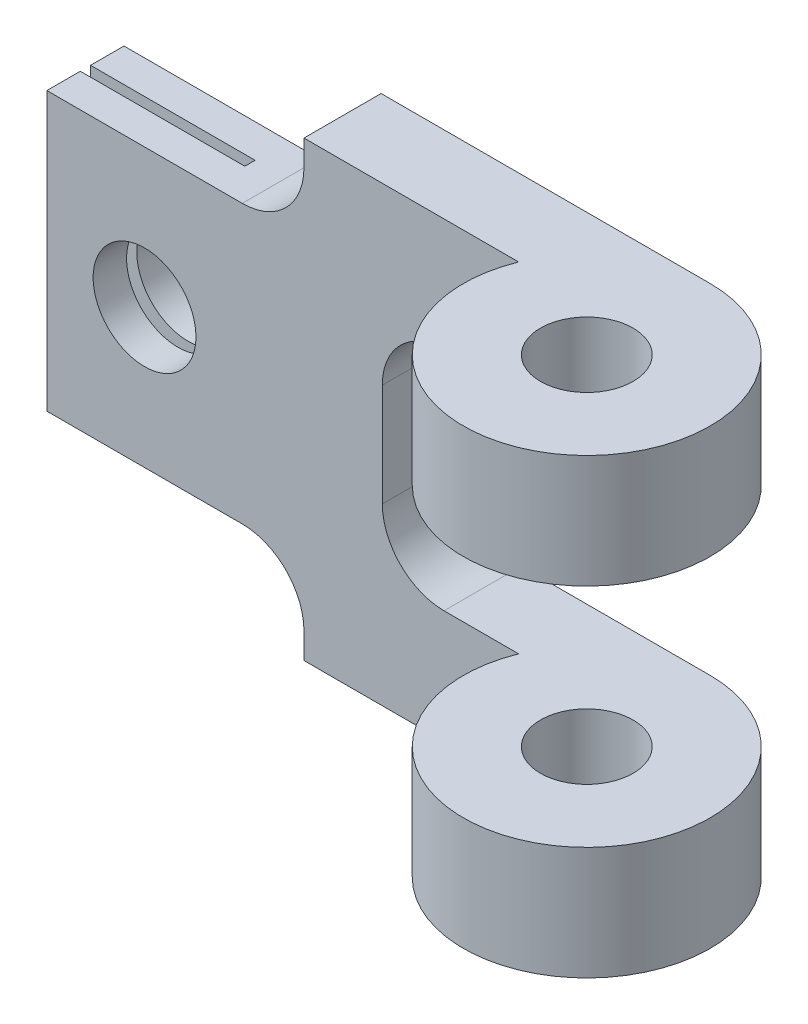
ISO-10303-21;
HEADER;
FILE_DESCRIPTION(('STEP AP214'),'2;1');
FILE_NAME('part.step','',(''),(''),'','','');
FILE_SCHEMA(('AUTOMOTIVE_DESIGN { 1 0 10303 214 1 1 1 1 }'));
ENDSEC;
DATA;
#1=APPLICATION_CONTEXT('core data for automotive mechanical design processes');
#2=APPLICATION_PROTOCOL_DEFINITION('international standard','automotive_design',2000,#1);
#3=PRODUCT_CONTEXT('',#1,'mechanical');
#4=PRODUCT('Part','Part','',(#3));
#5=PRODUCT_RELATED_PRODUCT_CATEGORY('part','',(#4));
#6=PRODUCT_DEFINITION_FORMATION('','',#4);
#7=PRODUCT_DEFINITION_CONTEXT('part definition',#1,'design');
#8=PRODUCT_DEFINITION('design','',#6,#7);
#9=PRODUCT_DEFINITION_SHAPE('','',#8);
#10=(LENGTH_UNIT() NAMED_UNIT(*) SI_UNIT(.MILLI.,.METRE.));
#11=(NAMED_UNIT(*) PLANE_ANGLE_UNIT() SI_UNIT($,.RADIAN.));
#12=(NAMED_UNIT(*) SI_UNIT($,.STERADIAN.) SOLID_ANGLE_UNIT());
#13=UNCERTAINTY_MEASURE_WITH_UNIT(LENGTH_MEASURE(1.E-05),#10,'distance_accuracy_value','');
#14=(GEOMETRIC_REPRESENTATION_CONTEXT(3) GLOBAL_UNCERTAINTY_ASSIGNED_CONTEXT((#13)) GLOBAL_UNIT_ASSIGNED_CONTEXT((#10,
#11,#12)) REPRESENTATION_CONTEXT('',''));
#15=CARTESIAN_POINT('',(0.,0.,0.));
#16=DIRECTION('',(0.,0.,1.));
#17=DIRECTION('',(1.,0.,0.));
#18=AXIS2_PLACEMENT_3D('',#15,#16,#17);
#19=CARTESIAN_POINT('',(-50.,-71.,15.));
#20=DIRECTION('',(-1.,0.,0.));
#21=DIRECTION('',(0.,0.,1.));
#22=AXIS2_PLACEMENT_3D('',#19,#20,#21);
#23=PLANE('',#22);
#24=DIRECTION('',(0.,1.,0.));
#25=VECTOR('',#24,1.);
#26=CARTESIAN_POINT('',(-50.,-72.,6.5));
#27=LINE('',#26,#25);
#28=CARTESIAN_POINT('',(-50.,-71.,6.5));
#29=VERTEX_POINT('',#28);
#30=CARTESIAN_POINT('',(-50.,-17.,6.5));
#31=VERTEX_POINT('',#30);
#32=EDGE_CURVE('E330',#29,#31,#27,.T.);
#33=ORIENTED_EDGE('',*,*,#32,.T.);
#34=DIRECTION('',(0.,0.,-1.));
#35=VECTOR('',#34,1.);
#36=CARTESIAN_POINT('',(-50.,-17.,15.));
#37=LINE('',#36,#35);
#38=CARTESIAN_POINT('',(-50.,-17.,0.));
#39=VERTEX_POINT('',#38);
#40=EDGE_CURVE('E206',#31,#39,#37,.T.);
#41=ORIENTED_EDGE('',*,*,#40,.T.);
#42=DIRECTION('',(0.,1.,0.));
#43=VECTOR('',#42,1.);
#44=CARTESIAN_POINT('',(-50.,-71.,0.));
#45=LINE('',#44,#43);
#46=CARTESIAN_POINT('',(-50.,-71.,0.));
#47=VERTEX_POINT('',#46);
#48=EDGE_CURVE('E332',#47,#39,#45,.T.);
#49=ORIENTED_EDGE('',*,*,#48,.F.);
#50=DIRECTION('',(0.,0.,-1.));
#51=VECTOR('',#50,1.);
#52=CARTESIAN_POINT('',(-50.,-71.,15.));
#53=LINE('',#52,#51);
#54=EDGE_CURVE('E219',#29,#47,#53,.T.);
#55=ORIENTED_EDGE('',*,*,#54,.F.);
#56=EDGE_LOOP('',(#33,#41,#49,#55));
#57=FACE_BOUND('',#56,.T.);
#58=ADVANCED_FACE('F44',(#57),#23,.T.);
#59=CARTESIAN_POINT('',(0.,0.,15.));
#60=DIRECTION('',(1.,0.,0.));
#61=DIRECTION('',(0.,0.,-1.));
#62=AXIS2_PLACEMENT_3D('',#59,#60,#61);
#63=PLANE('',#62);
#64=DIRECTION('',(0.,0.,-1.));
#65=VECTOR('',#64,1.);
#66=CARTESIAN_POINT('',(0.,-83.0000000000001,15.));
#67=LINE('',#66,#65);
#68=CARTESIAN_POINT('',(0.,-83.,15.));
#69=VERTEX_POINT('',#68);
#70=CARTESIAN_POINT('',(0.,-83.0000000000001,0.));
#71=VERTEX_POINT('',#70);
#72=EDGE_CURVE('E218',#69,#71,#67,.T.);
#73=ORIENTED_EDGE('',*,*,#72,.T.);
#74=DIRECTION('',(0.,-1.,0.));
#75=VECTOR('',#74,1.);
#76=CARTESIAN_POINT('',(0.,0.,0.));
#77=LINE('',#76,#75);
#78=CARTESIAN_POINT('',(0.,-88.,0.));
#79=VERTEX_POINT('',#78);
#80=EDGE_CURVE('E239',#71,#79,#77,.T.);
#81=ORIENTED_EDGE('',*,*,#80,.T.);
#82=DIRECTION('',(0.,0.,-1.));
#83=VECTOR('',#82,1.);
#84=CARTESIAN_POINT('',(0.,-88.,15.));
#85=LINE('',#84,#83);
#86=CARTESIAN_POINT('',(0.,-88.,15.));
#87=VERTEX_POINT('',#86);
#88=EDGE_CURVE('E294',#87,#79,#85,.T.);
#89=ORIENTED_EDGE('',*,*,#88,.F.);
#90=DIRECTION('',(0.,-1.,0.));
#91=VECTOR('',#90,1.);
#92=CARTESIAN_POINT('',(0.,0.,15.));
#93=LINE('',#92,#91);
#94=EDGE_CURVE('E68',#69,#87,#93,.T.);
#95=ORIENTED_EDGE('',*,*,#94,.F.);
#96=EDGE_LOOP('',(#73,#81,#89,#95));
#97=FACE_BOUND('',#96,.T.);
#98=ADVANCED_FACE('F395',(#97),#63,.F.);
#99=CARTESIAN_POINT('',(0.,0.,0.));
#100=VERTEX_POINT('',#99);
#101=CARTESIAN_POINT('',(0.,-5.,0.));
#102=VERTEX_POINT('',#101);
#103=EDGE_CURVE('E256',#100,#102,#77,.T.);
#104=ORIENTED_EDGE('',*,*,#103,.T.);
#105=DIRECTION('',(0.,0.,-1.));
#106=VECTOR('',#105,1.);
#107=CARTESIAN_POINT('',(0.,-4.99999999999992,15.));
#108=LINE('',#107,#106);
#109=CARTESIAN_POINT('',(0.,-5.,15.));
#110=VERTEX_POINT('',#109);
#111=EDGE_CURVE('E208',#110,#102,#108,.T.);
#112=ORIENTED_EDGE('',*,*,#111,.F.);
#113=CARTESIAN_POINT('',(0.,0.,15.));
#114=VERTEX_POINT('',#113);
#115=EDGE_CURVE('E241',#114,#110,#93,.T.);
#116=ORIENTED_EDGE('',*,*,#115,.F.);
#117=DIRECTION('',(0.,0.,-1.));
#118=VECTOR('',#117,1.);
#119=CARTESIAN_POINT('',(0.,0.,15.));
#120=LINE('',#119,#118);
#121=EDGE_CURVE('E259',#114,#100,#120,.T.);
#122=ORIENTED_EDGE('',*,*,#121,.T.);
#123=EDGE_LOOP('',(#104,#112,#116,#122));
#124=FACE_BOUND('',#123,.T.);
#125=ADVANCED_FACE('F50',(#124),#63,.F.);
#126=CARTESIAN_POINT('',(0.,-88.,15.));
#127=DIRECTION('',(0.,1.,0.));
#128=DIRECTION('',(0.,0.,1.));
#129=AXIS2_PLACEMENT_3D('',#126,#127,#128);
#130=PLANE('',#129);
#131=CARTESIAN_POINT('',(64.,-88.,24.));
#132=DIRECTION('',(0.,1.,0.));
#133=DIRECTION('',(0.,0.,1.));
#134=AXIS2_PLACEMENT_3D('',#131,#132,#133);
#135=CIRCLE('',#134,9.);
#136=CARTESIAN_POINT('',(64.,-88.,33.));
#137=VERTEX_POINT('',#136);
#138=EDGE_CURVE('E412',#137,#137,#135,.T.);
#139=ORIENTED_EDGE('',*,*,#138,.T.);
#140=EDGE_LOOP('',(#139));
#141=FACE_BOUND('',#140,.T.);
#142=DIRECTION('',(1.,0.,0.));
#143=VECTOR('',#142,1.);
#144=CARTESIAN_POINT('',(0.,-88.,0.));
#145=LINE('',#144,#143);
#146=CARTESIAN_POINT('',(64.,-88.,0.));
#147=VERTEX_POINT('',#146);
#148=EDGE_CURVE('E264',#79,#147,#145,.T.);
#149=ORIENTED_EDGE('',*,*,#148,.T.);
#150=CARTESIAN_POINT('',(64.,-88.,24.));
#151=DIRECTION('',(0.,-1.,0.));
#152=DIRECTION('',(0.,0.,-1.));
#153=AXIS2_PLACEMENT_3D('',#150,#151,#152);
#154=CIRCLE('',#153,24.);
#155=CARTESIAN_POINT('',(41.751404538713,-88.,15.));
#156=VERTEX_POINT('',#155);
#157=EDGE_CURVE('E228',#147,#156,#154,.T.);
#158=ORIENTED_EDGE('',*,*,#157,.T.);
#159=DIRECTION('',(1.,0.,0.));
#160=VECTOR('',#159,1.);
#161=CARTESIAN_POINT('',(0.,-88.,15.));
#162=LINE('',#161,#160);
#163=EDGE_CURVE('E242',#87,#156,#162,.T.);
#164=ORIENTED_EDGE('',*,*,#163,.F.);
#165=ORIENTED_EDGE('',*,*,#88,.T.);
#166=EDGE_LOOP('',(#149,#158,#164,#165));
#167=FACE_BOUND('',#166,.T.);
#168=ADVANCED_FACE('F394',(#141,#167),#130,.F.);
#169=CARTESIAN_POINT('',(64.,-66.,15.));
#170=DIRECTION('',(0.,-1.,0.));
#171=DIRECTION('',(0.,0.,-1.));
#172=AXIS2_PLACEMENT_3D('',#169,#170,#171);
#173=PLANE('',#172);
#174=CARTESIAN_POINT('',(64.,-66.,24.));
#175=DIRECTION('',(0.,-1.,0.));
#176=DIRECTION('',(0.,0.,-1.));
#177=AXIS2_PLACEMENT_3D('',#174,#175,#176);
#178=CIRCLE('',#177,9.);
#179=CARTESIAN_POINT('',(64.,-66.,33.));
#180=VERTEX_POINT('',#179);
#181=EDGE_CURVE('E420',#180,#180,#178,.T.);
#182=ORIENTED_EDGE('',*,*,#181,.T.);
#183=EDGE_LOOP('',(#182));
#184=FACE_BOUND('',#183,.T.);
#185=CARTESIAN_POINT('',(64.,-66.,24.));
#186=DIRECTION('',(0.,-1.,0.));
#187=DIRECTION('',(0.,0.,-1.));
#188=AXIS2_PLACEMENT_3D('',#185,#186,#187);
#189=CIRCLE('',#188,24.);
#190=CARTESIAN_POINT('',(64.,-66.,0.));
#191=VERTEX_POINT('',#190);
#192=CARTESIAN_POINT('',(41.751404538713,-66.,15.));
#193=VERTEX_POINT('',#192);
#194=EDGE_CURVE('E224',#191,#193,#189,.T.);
#195=ORIENTED_EDGE('',*,*,#194,.F.);
#196=DIRECTION('',(-1.,0.,0.));
#197=VECTOR('',#196,1.);
#198=CARTESIAN_POINT('',(64.,-66.,0.));
#199=LINE('',#198,#197);
#200=CARTESIAN_POINT('',(27.2400000000001,-66.,0.));
#201=VERTEX_POINT('',#200);
#202=EDGE_CURVE('E267',#191,#201,#199,.T.);
#203=ORIENTED_EDGE('',*,*,#202,.T.);
#204=DIRECTION('',(0.,0.,-1.));
#205=VECTOR('',#204,1.);
#206=CARTESIAN_POINT('',(27.2400000000001,-66.,15.));
#207=LINE('',#206,#205);
#208=CARTESIAN_POINT('',(27.2400000000001,-66.,15.));
#209=VERTEX_POINT('',#208);
#210=EDGE_CURVE('E292',#209,#201,#207,.T.);
#211=ORIENTED_EDGE('',*,*,#210,.F.);
#212=DIRECTION('',(-1.,0.,0.));
#213=VECTOR('',#212,1.);
#214=CARTESIAN_POINT('',(64.,-66.,15.));
#215=LINE('',#214,#213);
#216=EDGE_CURVE('E246',#193,#209,#215,.T.);
#217=ORIENTED_EDGE('',*,*,#216,.F.);
#218=EDGE_LOOP('',(#195,#203,#211,#217));
#219=FACE_BOUND('',#218,.T.);
#220=ADVANCED_FACE('F389',(#184,#219),#173,.F.);
#221=CARTESIAN_POINT('',(27.24,-54.,15.));
#222=DIRECTION('',(0.,0.,-1.));
#223=DIRECTION('',(-1.,0.,0.));
#224=AXIS2_PLACEMENT_3D('',#221,#222,#223);
#225=CYLINDRICAL_SURFACE('',#224,12.);
#226=CARTESIAN_POINT('',(27.24,-54.,0.));
#227=DIRECTION('',(0.,0.,-1.));
#228=DIRECTION('',(1.,0.,0.));
#229=AXIS2_PLACEMENT_3D('',#226,#227,#228);
#230=CIRCLE('',#229,12.);
#231=CARTESIAN_POINT('',(15.24,-53.9999999999999,0.));
#232=VERTEX_POINT('',#231);
#233=EDGE_CURVE('E270',#201,#232,#230,.T.);
#234=ORIENTED_EDGE('',*,*,#233,.T.);
#235=DIRECTION('',(0.,0.,-1.));
#236=VECTOR('',#235,1.);
#237=CARTESIAN_POINT('',(15.24,-53.9999999999999,15.));
#238=LINE('',#237,#236);
#239=CARTESIAN_POINT('',(15.24,-53.9999999999999,15.));
#240=VERTEX_POINT('',#239);
#241=EDGE_CURVE('E286',#240,#232,#238,.T.);
#242=ORIENTED_EDGE('',*,*,#241,.F.);
#243=CARTESIAN_POINT('',(27.24,-54.,15.));
#244=DIRECTION('',(0.,0.,-1.));
#245=DIRECTION('',(1.,0.,0.));
#246=AXIS2_PLACEMENT_3D('',#243,#244,#245);
#247=CIRCLE('',#246,12.);
#248=EDGE_CURVE('E247',#209,#240,#247,.T.);
#249=ORIENTED_EDGE('',*,*,#248,.F.);
#250=ORIENTED_EDGE('',*,*,#210,.T.);
#251=EDGE_LOOP('',(#234,#242,#249,#250));
#252=FACE_BOUND('',#251,.T.);
#253=ADVANCED_FACE('F377',(#252),#225,.F.);
#254=CARTESIAN_POINT('',(15.24,-53.9999999999999,15.));
#255=DIRECTION('',(-1.,0.,0.));
#256=DIRECTION('',(0.,0.,1.));
#257=AXIS2_PLACEMENT_3D('',#254,#255,#256);
#258=PLANE('',#257);
#259=DIRECTION('',(0.,1.,0.));
#260=VECTOR('',#259,1.);
#261=CARTESIAN_POINT('',(15.24,-53.9999999999999,0.));
#262=LINE('',#261,#260);
#263=CARTESIAN_POINT('',(15.24,-34.0000000000001,0.));
#264=VERTEX_POINT('',#263);
#265=EDGE_CURVE('E268',#232,#264,#262,.T.);
#266=ORIENTED_EDGE('',*,*,#265,.T.);
#267=DIRECTION('',(0.,0.,-1.));
#268=VECTOR('',#267,1.);
#269=CARTESIAN_POINT('',(15.24,-34.0000000000001,15.));
#270=LINE('',#269,#268);
#271=CARTESIAN_POINT('',(15.24,-34.0000000000001,15.));
#272=VERTEX_POINT('',#271);
#273=EDGE_CURVE('E287',#272,#264,#270,.T.);
#274=ORIENTED_EDGE('',*,*,#273,.F.);
#275=DIRECTION('',(0.,1.,0.));
#276=VECTOR('',#275,1.);
#277=CARTESIAN_POINT('',(15.24,-53.9999999999999,15.));
#278=LINE('',#277,#276);
#279=EDGE_CURVE('E249',#240,#272,#278,.T.);
#280=ORIENTED_EDGE('',*,*,#279,.F.);
#281=ORIENTED_EDGE('',*,*,#241,.T.);
#282=EDGE_LOOP('',(#266,#274,#280,#281));
#283=FACE_BOUND('',#282,.T.);
#284=ADVANCED_FACE('F372',(#283),#258,.F.);
#285=CARTESIAN_POINT('',(27.24,-34.,15.));
#286=DIRECTION('',(0.,0.,-1.));
#287=DIRECTION('',(-1.,0.,0.));
#288=AXIS2_PLACEMENT_3D('',#285,#286,#287);
#289=CYLINDRICAL_SURFACE('',#288,12.);
#290=CARTESIAN_POINT('',(27.24,-34.,0.));
#291=DIRECTION('',(0.,0.,-1.));
#292=DIRECTION('',(1.,0.,0.));
#293=AXIS2_PLACEMENT_3D('',#290,#291,#292);
#294=CIRCLE('',#293,12.);
#295=CARTESIAN_POINT('',(27.2400000000001,-22.,0.));
#296=VERTEX_POINT('',#295);
#297=EDGE_CURVE('E275',#264,#296,#294,.T.);
#298=ORIENTED_EDGE('',*,*,#297,.T.);
#299=DIRECTION('',(0.,0.,-1.));
#300=VECTOR('',#299,1.);
#301=CARTESIAN_POINT('',(27.2400000000001,-22.,15.));
#302=LINE('',#301,#300);
#303=CARTESIAN_POINT('',(27.2400000000001,-22.,15.));
#304=VERTEX_POINT('',#303);
#305=EDGE_CURVE('E285',#304,#296,#302,.T.);
#306=ORIENTED_EDGE('',*,*,#305,.F.);
#307=CARTESIAN_POINT('',(27.24,-34.,15.));
#308=DIRECTION('',(0.,0.,-1.));
#309=DIRECTION('',(1.,0.,0.));
#310=AXIS2_PLACEMENT_3D('',#307,#308,#309);
#311=CIRCLE('',#310,12.);
#312=EDGE_CURVE('E255',#272,#304,#311,.T.);
#313=ORIENTED_EDGE('',*,*,#312,.F.);
#314=ORIENTED_EDGE('',*,*,#273,.T.);
#315=EDGE_LOOP('',(#298,#306,#313,#314));
#316=FACE_BOUND('',#315,.T.);
#317=ADVANCED_FACE('F367',(#316),#289,.F.);
#318=CARTESIAN_POINT('',(27.2400000000001,-22.,15.));
#319=DIRECTION('',(0.,1.,0.));
#320=DIRECTION('',(0.,0.,1.));
#321=AXIS2_PLACEMENT_3D('',#318,#319,#320);
#322=PLANE('',#321);
#323=CARTESIAN_POINT('',(64.,-22.,24.));
#324=DIRECTION('',(0.,1.,0.));
#325=DIRECTION('',(0.,0.,1.));
#326=AXIS2_PLACEMENT_3D('',#323,#324,#325);
#327=CIRCLE('',#326,9.);
#328=CARTESIAN_POINT('',(64.,-22.,33.));
#329=VERTEX_POINT('',#328);
#330=EDGE_CURVE('E423',#329,#329,#327,.T.);
#331=ORIENTED_EDGE('',*,*,#330,.T.);
#332=EDGE_LOOP('',(#331));
#333=FACE_BOUND('',#332,.T.);
#334=DIRECTION('',(1.,0.,0.));
#335=VECTOR('',#334,1.);
#336=CARTESIAN_POINT('',(27.2400000000001,-22.,0.));
#337=LINE('',#336,#335);
#338=CARTESIAN_POINT('',(64.,-22.,0.));
#339=VERTEX_POINT('',#338);
#340=EDGE_CURVE('E274',#296,#339,#337,.T.);
#341=ORIENTED_EDGE('',*,*,#340,.T.);
#342=CARTESIAN_POINT('',(64.,-22.,24.));
#343=DIRECTION('',(0.,1.,0.));
#344=DIRECTION('',(0.,0.,1.));
#345=AXIS2_PLACEMENT_3D('',#342,#343,#344);
#346=CIRCLE('',#345,24.);
#347=CARTESIAN_POINT('',(41.751404538713,-22.,15.));
#348=VERTEX_POINT('',#347);
#349=EDGE_CURVE('E235',#348,#339,#346,.T.);
#350=ORIENTED_EDGE('',*,*,#349,.F.);
#351=DIRECTION('',(1.,0.,0.));
#352=VECTOR('',#351,1.);
#353=CARTESIAN_POINT('',(27.2400000000001,-22.,15.));
#354=LINE('',#353,#352);
#355=EDGE_CURVE('E251',#304,#348,#354,.T.);
#356=ORIENTED_EDGE('',*,*,#355,.F.);
#357=ORIENTED_EDGE('',*,*,#305,.T.);
#358=EDGE_LOOP('',(#341,#350,#356,#357));
#359=FACE_BOUND('',#358,.T.);
#360=ADVANCED_FACE('F361',(#333,#359),#322,.F.);
#361=CARTESIAN_POINT('',(0.,0.,15.));
#362=DIRECTION('',(0.,-1.,0.));
#363=DIRECTION('',(0.,0.,-1.));
#364=AXIS2_PLACEMENT_3D('',#361,#362,#363);
#365=PLANE('',#364);
#366=CARTESIAN_POINT('',(64.,0.,24.));
#367=DIRECTION('',(0.,1.,0.));
#368=DIRECTION('',(0.,0.,1.));
#369=AXIS2_PLACEMENT_3D('',#366,#367,#368);
#370=CIRCLE('',#369,9.);
#371=CARTESIAN_POINT('',(64.,0.,33.));
#372=VERTEX_POINT('',#371);
#373=EDGE_CURVE('E425',#372,#372,#370,.T.);
#374=ORIENTED_EDGE('',*,*,#373,.F.);
#375=EDGE_LOOP('',(#374));
#376=FACE_BOUND('',#375,.T.);
#377=CARTESIAN_POINT('',(64.,0.,24.));
#378=DIRECTION('',(0.,1.,0.));
#379=DIRECTION('',(0.,0.,1.));
#380=AXIS2_PLACEMENT_3D('',#377,#378,#379);
#381=CIRCLE('',#380,24.);
#382=CARTESIAN_POINT('',(41.751404538713,0.,15.));
#383=VERTEX_POINT('',#382);
#384=CARTESIAN_POINT('',(64.,0.,0.));
#385=VERTEX_POINT('',#384);
#386=EDGE_CURVE('E233',#383,#385,#381,.T.);
#387=ORIENTED_EDGE('',*,*,#386,.T.);
#388=DIRECTION('',(-1.,0.,0.));
#389=VECTOR('',#388,1.);
#390=CARTESIAN_POINT('',(0.,0.,0.));
#391=LINE('',#390,#389);
#392=EDGE_CURVE('E276',#385,#100,#391,.T.);
#393=ORIENTED_EDGE('',*,*,#392,.T.);
#394=ORIENTED_EDGE('',*,*,#121,.F.);
#395=DIRECTION('',(-1.,0.,0.));
#396=VECTOR('',#395,1.);
#397=CARTESIAN_POINT('',(0.,0.,15.));
#398=LINE('',#397,#396);
#399=EDGE_CURVE('E257',#383,#114,#398,.T.);
#400=ORIENTED_EDGE('',*,*,#399,.F.);
#401=EDGE_LOOP('',(#387,#393,#394,#400));
#402=FACE_BOUND('',#401,.T.);
#403=ADVANCED_FACE('F351',(#376,#402),#365,.F.);
#404=CARTESIAN_POINT('',(27.24,-54.,15.));
#405=DIRECTION('',(0.,0.,1.));
#406=DIRECTION('',(1.,0.,0.));
#407=AXIS2_PLACEMENT_3D('',#404,#405,#406);
#408=PLANE('',#407);
#409=CARTESIAN_POINT('',(-31.,-44.,15.));
#410=DIRECTION('',(0.,0.,1.));
#411=DIRECTION('',(1.,0.,0.));
#412=AXIS2_PLACEMENT_3D('',#409,#410,#411);
#413=CIRCLE('',#412,10.);
#414=CARTESIAN_POINT('',(-21.,-44.,15.));
#415=VERTEX_POINT('',#414);
#416=EDGE_CURVE('E411',#415,#415,#413,.T.);
#417=ORIENTED_EDGE('',*,*,#416,.F.);
#418=EDGE_LOOP('',(#417));
#419=FACE_BOUND('',#418,.T.);
#420=DIRECTION('',(0.,-1.,0.));
#421=VECTOR('',#420,1.);
#422=CARTESIAN_POINT('',(41.751404538713,-66.,15.));
#423=LINE('',#422,#421);
#424=EDGE_CURVE('E223',#193,#156,#423,.T.);
#425=ORIENTED_EDGE('',*,*,#424,.F.);
#426=ORIENTED_EDGE('',*,*,#216,.T.);
#427=ORIENTED_EDGE('',*,*,#248,.T.);
#428=ORIENTED_EDGE('',*,*,#279,.T.);
#429=ORIENTED_EDGE('',*,*,#312,.T.);
#430=ORIENTED_EDGE('',*,*,#355,.T.);
#431=DIRECTION('',(0.,1.,0.));
#432=VECTOR('',#431,1.);
#433=CARTESIAN_POINT('',(41.751404538713,-22.,15.));
#434=LINE('',#433,#432);
#435=EDGE_CURVE('E232',#383,#348,#434,.F.);
#436=ORIENTED_EDGE('',*,*,#435,.F.);
#437=ORIENTED_EDGE('',*,*,#399,.T.);
#438=ORIENTED_EDGE('',*,*,#115,.T.);
#439=CARTESIAN_POINT('',(-12.,-5.,15.));
#440=DIRECTION('',(0.,0.,1.));
#441=DIRECTION('',(-1.,0.,0.));
#442=AXIS2_PLACEMENT_3D('',#439,#440,#441);
#443=CIRCLE('',#442,12.);
#444=CARTESIAN_POINT('',(-12.0000000000001,-17.,15.));
#445=VERTEX_POINT('',#444);
#446=EDGE_CURVE('E222',#445,#110,#443,.T.);
#447=ORIENTED_EDGE('',*,*,#446,.F.);
#448=DIRECTION('',(1.,0.,0.));
#449=VECTOR('',#448,1.);
#450=CARTESIAN_POINT('',(-50.,-17.,15.));
#451=LINE('',#450,#449);
#452=CARTESIAN_POINT('',(-50.,-17.,15.));
#453=VERTEX_POINT('',#452);
#454=EDGE_CURVE('E314',#453,#445,#451,.T.);
#455=ORIENTED_EDGE('',*,*,#454,.F.);
#456=DIRECTION('',(0.,1.,0.));
#457=VECTOR('',#456,1.);
#458=CARTESIAN_POINT('',(-50.,-71.,15.));
#459=LINE('',#458,#457);
#460=CARTESIAN_POINT('',(-50.,-71.,15.));
#461=VERTEX_POINT('',#460);
#462=EDGE_CURVE('E207',#461,#453,#459,.T.);
#463=ORIENTED_EDGE('',*,*,#462,.F.);
#464=DIRECTION('',(-1.,0.,0.));
#465=VECTOR('',#464,1.);
#466=CARTESIAN_POINT('',(-12.0000000000001,-71.,15.));
#467=LINE('',#466,#465);
#468=CARTESIAN_POINT('',(-12.0000000000001,-71.,15.));
#469=VERTEX_POINT('',#468);
#470=EDGE_CURVE('E307',#469,#461,#467,.T.);
#471=ORIENTED_EDGE('',*,*,#470,.F.);
#472=CARTESIAN_POINT('',(-12.,-83.,15.));
#473=DIRECTION('',(0.,0.,1.));
#474=DIRECTION('',(-1.,0.,0.));
#475=AXIS2_PLACEMENT_3D('',#472,#473,#474);
#476=CIRCLE('',#475,12.);
#477=EDGE_CURVE('E319',#69,#469,#476,.T.);
#478=ORIENTED_EDGE('',*,*,#477,.F.);
#479=ORIENTED_EDGE('',*,*,#94,.T.);
#480=ORIENTED_EDGE('',*,*,#163,.T.);
#481=EDGE_LOOP('',(#425,#426,#427,#428,#429,#430,#436,#437,#438,#447,#455,#463,#471,#478,#479,#480));
#482=FACE_BOUND('',#481,.T.);
#483=ADVANCED_FACE('F311',(#419,#482),#408,.T.);
#484=CARTESIAN_POINT('',(27.24,-54.,0.));
#485=DIRECTION('',(0.,0.,1.));
#486=DIRECTION('',(1.,0.,0.));
#487=AXIS2_PLACEMENT_3D('',#484,#485,#486);
#488=PLANE('',#487);
#489=CARTESIAN_POINT('',(-31.,-44.,0.));
#490=DIRECTION('',(0.,0.,1.));
#491=DIRECTION('',(1.,0.,0.));
#492=AXIS2_PLACEMENT_3D('',#489,#490,#491);
#493=CIRCLE('',#492,10.);
#494=CARTESIAN_POINT('',(-21.,-44.,0.));
#495=VERTEX_POINT('',#494);
#496=EDGE_CURVE('E202',#495,#495,#493,.T.);
#497=ORIENTED_EDGE('',*,*,#496,.T.);
#498=EDGE_LOOP('',(#497));
#499=FACE_BOUND('',#498,.T.);
#500=ORIENTED_EDGE('',*,*,#103,.F.);
#501=ORIENTED_EDGE('',*,*,#392,.F.);
#502=DIRECTION('',(0.,1.,0.));
#503=VECTOR('',#502,1.);
#504=CARTESIAN_POINT('',(64.,-22.,0.));
#505=LINE('',#504,#503);
#506=EDGE_CURVE('E277',#339,#385,#505,.T.);
#507=ORIENTED_EDGE('',*,*,#506,.F.);
#508=ORIENTED_EDGE('',*,*,#340,.F.);
#509=ORIENTED_EDGE('',*,*,#297,.F.);
#510=ORIENTED_EDGE('',*,*,#265,.F.);
#511=ORIENTED_EDGE('',*,*,#233,.F.);
#512=ORIENTED_EDGE('',*,*,#202,.F.);
#513=DIRECTION('',(0.,1.,0.));
#514=VECTOR('',#513,1.);
#515=CARTESIAN_POINT('',(64.,-88.,0.));
#516=LINE('',#515,#514);
#517=EDGE_CURVE('E265',#147,#191,#516,.T.);
#518=ORIENTED_EDGE('',*,*,#517,.F.);
#519=ORIENTED_EDGE('',*,*,#148,.F.);
#520=ORIENTED_EDGE('',*,*,#80,.F.);
#521=CARTESIAN_POINT('',(-12.,-83.,0.));
#522=DIRECTION('',(0.,0.,1.));
#523=DIRECTION('',(-1.,0.,0.));
#524=AXIS2_PLACEMENT_3D('',#521,#522,#523);
#525=CIRCLE('',#524,12.);
#526=CARTESIAN_POINT('',(-12.0000000000001,-71.,0.));
#527=VERTEX_POINT('',#526);
#528=EDGE_CURVE('E321',#71,#527,#525,.T.);
#529=ORIENTED_EDGE('',*,*,#528,.T.);
#530=DIRECTION('',(-1.,0.,0.));
#531=VECTOR('',#530,1.);
#532=CARTESIAN_POINT('',(-12.0000000000001,-71.,0.));
#533=LINE('',#532,#531);
#534=EDGE_CURVE('E326',#527,#47,#533,.T.);
#535=ORIENTED_EDGE('',*,*,#534,.T.);
#536=ORIENTED_EDGE('',*,*,#48,.T.);
#537=DIRECTION('',(1.,0.,0.));
#538=VECTOR('',#537,1.);
#539=CARTESIAN_POINT('',(-50.,-17.,0.));
#540=LINE('',#539,#538);
#541=CARTESIAN_POINT('',(-12.0000000000001,-17.,0.));
#542=VERTEX_POINT('',#541);
#543=EDGE_CURVE('E331',#39,#542,#540,.T.);
#544=ORIENTED_EDGE('',*,*,#543,.T.);
#545=CARTESIAN_POINT('',(-12.,-5.,0.));
#546=DIRECTION('',(0.,0.,1.));
#547=DIRECTION('',(-1.,0.,0.));
#548=AXIS2_PLACEMENT_3D('',#545,#546,#547);
#549=CIRCLE('',#548,12.);
#550=EDGE_CURVE('E340',#542,#102,#549,.T.);
#551=ORIENTED_EDGE('',*,*,#550,.T.);
#552=EDGE_LOOP('',(#500,#501,#507,#508,#509,#510,#511,#512,#518,#519,#520,#529,#535,#536,#544,#551));
#553=FACE_BOUND('',#552,.T.);
#554=ADVANCED_FACE('F346',(#499,#553),#488,.F.);
#555=CARTESIAN_POINT('',(64.,-22.,24.));
#556=DIRECTION('',(0.,1.,0.));
#557=DIRECTION('',(0.,0.,1.));
#558=AXIS2_PLACEMENT_3D('',#555,#556,#557);
#559=CYLINDRICAL_SURFACE('',#558,24.);
#560=ORIENTED_EDGE('',*,*,#386,.F.);
#561=ORIENTED_EDGE('',*,*,#435,.T.);
#562=ORIENTED_EDGE('',*,*,#349,.T.);
#563=ORIENTED_EDGE('',*,*,#506,.T.);
#564=EDGE_LOOP('',(#560,#561,#562,#563));
#565=FACE_BOUND('',#564,.T.);
#566=ADVANCED_FACE('F360',(#565),#559,.T.);
#567=CARTESIAN_POINT('',(64.,-66.,24.));
#568=DIRECTION('',(0.,-1.,0.));
#569=DIRECTION('',(0.,0.,-1.));
#570=AXIS2_PLACEMENT_3D('',#567,#568,#569);
#571=CYLINDRICAL_SURFACE('',#570,24.);
#572=ORIENTED_EDGE('',*,*,#194,.T.);
#573=ORIENTED_EDGE('',*,*,#424,.T.);
#574=ORIENTED_EDGE('',*,*,#157,.F.);
#575=ORIENTED_EDGE('',*,*,#517,.T.);
#576=EDGE_LOOP('',(#572,#573,#574,#575));
#577=FACE_BOUND('',#576,.T.);
#578=ADVANCED_FACE('F387',(#577),#571,.T.);
#579=CARTESIAN_POINT('',(-12.,-5.,15.));
#580=DIRECTION('',(0.,0.,-1.));
#581=DIRECTION('',(-1.,0.,0.));
#582=AXIS2_PLACEMENT_3D('',#579,#580,#581);
#583=CYLINDRICAL_SURFACE('',#582,12.);
#584=ORIENTED_EDGE('',*,*,#550,.F.);
#585=DIRECTION('',(0.,0.,-1.));
#586=VECTOR('',#585,1.);
#587=CARTESIAN_POINT('',(-12.0000000000001,-17.,15.));
#588=LINE('',#587,#586);
#589=EDGE_CURVE('E210',#445,#542,#588,.T.);
#590=ORIENTED_EDGE('',*,*,#589,.F.);
#591=ORIENTED_EDGE('',*,*,#446,.T.);
#592=ORIENTED_EDGE('',*,*,#111,.T.);
#593=EDGE_LOOP('',(#584,#590,#591,#592));
#594=FACE_BOUND('',#593,.T.);
#595=ADVANCED_FACE('F345',(#594),#583,.F.);
#596=CARTESIAN_POINT('',(-50.,-17.,15.));
#597=DIRECTION('',(0.,1.,0.));
#598=DIRECTION('',(0.,0.,1.));
#599=AXIS2_PLACEMENT_3D('',#596,#597,#598);
#600=PLANE('',#599);
#601=DIRECTION('',(-1.,0.,0.));
#602=VECTOR('',#601,1.);
#603=CARTESIAN_POINT('',(-50.,-17.,6.5));
#604=LINE('',#603,#602);
#605=CARTESIAN_POINT('',(-18.,-17.,6.5));
#606=VERTEX_POINT('',#605);
#607=EDGE_CURVE('E192',#606,#31,#604,.T.);
#608=ORIENTED_EDGE('',*,*,#607,.F.);
#609=DIRECTION('',(0.,0.,-1.));
#610=VECTOR('',#609,1.);
#611=CARTESIAN_POINT('',(-18.,-17.,6.5));
#612=LINE('',#611,#610);
#613=CARTESIAN_POINT('',(-18.,-17.,8.5));
#614=VERTEX_POINT('',#613);
#615=EDGE_CURVE('E197',#614,#606,#612,.T.);
#616=ORIENTED_EDGE('',*,*,#615,.F.);
#617=DIRECTION('',(1.,0.,0.));
#618=VECTOR('',#617,1.);
#619=CARTESIAN_POINT('',(-18.,-17.,8.5));
#620=LINE('',#619,#618);
#621=CARTESIAN_POINT('',(-50.,-17.,8.5));
#622=VERTEX_POINT('',#621);
#623=EDGE_CURVE('E183',#622,#614,#620,.T.);
#624=ORIENTED_EDGE('',*,*,#623,.F.);
#625=EDGE_CURVE('E196',#453,#622,#37,.T.);
#626=ORIENTED_EDGE('',*,*,#625,.F.);
#627=ORIENTED_EDGE('',*,*,#454,.T.);
#628=ORIENTED_EDGE('',*,*,#589,.T.);
#629=ORIENTED_EDGE('',*,*,#543,.F.);
#630=ORIENTED_EDGE('',*,*,#40,.F.);
#631=EDGE_LOOP('',(#608,#616,#624,#626,#627,#628,#629,#630));
#632=FACE_BOUND('',#631,.T.);
#633=ADVANCED_FACE('F193',(#632),#600,.T.);
#634=DIRECTION('',(0.,1.,0.));
#635=VECTOR('',#634,1.);
#636=CARTESIAN_POINT('',(-50.,-72.,8.5));
#637=LINE('',#636,#635);
#638=CARTESIAN_POINT('',(-50.,-71.,8.5));
#639=VERTEX_POINT('',#638);
#640=EDGE_CURVE('E181',#639,#622,#637,.T.);
#641=ORIENTED_EDGE('',*,*,#640,.F.);
#642=EDGE_CURVE('E215',#461,#639,#53,.T.);
#643=ORIENTED_EDGE('',*,*,#642,.F.);
#644=ORIENTED_EDGE('',*,*,#462,.T.);
#645=ORIENTED_EDGE('',*,*,#625,.T.);
#646=EDGE_LOOP('',(#641,#643,#644,#645));
#647=FACE_BOUND('',#646,.T.);
#648=ADVANCED_FACE('F201',(#647),#23,.T.);
#649=CARTESIAN_POINT('',(-12.0000000000001,-71.,15.));
#650=DIRECTION('',(0.,-1.,0.));
#651=DIRECTION('',(0.,0.,-1.));
#652=AXIS2_PLACEMENT_3D('',#649,#650,#651);
#653=PLANE('',#652);
#654=DIRECTION('',(1.,0.,0.));
#655=VECTOR('',#654,1.);
#656=CARTESIAN_POINT('',(-12.0000000000001,-71.,6.5));
#657=LINE('',#656,#655);
#658=CARTESIAN_POINT('',(-18.,-71.,6.5));
#659=VERTEX_POINT('',#658);
#660=EDGE_CURVE('E11',#29,#659,#657,.T.);
#661=ORIENTED_EDGE('',*,*,#660,.F.);
#662=ORIENTED_EDGE('',*,*,#54,.T.);
#663=ORIENTED_EDGE('',*,*,#534,.F.);
#664=DIRECTION('',(0.,0.,-1.));
#665=VECTOR('',#664,1.);
#666=CARTESIAN_POINT('',(-12.0000000000001,-71.,15.));
#667=LINE('',#666,#665);
#668=EDGE_CURVE('E216',#469,#527,#667,.T.);
#669=ORIENTED_EDGE('',*,*,#668,.F.);
#670=ORIENTED_EDGE('',*,*,#470,.T.);
#671=ORIENTED_EDGE('',*,*,#642,.T.);
#672=DIRECTION('',(-1.,0.,0.));
#673=VECTOR('',#672,1.);
#674=CARTESIAN_POINT('',(-12.0000000000001,-71.,8.5));
#675=LINE('',#674,#673);
#676=CARTESIAN_POINT('',(-18.,-71.,8.5));
#677=VERTEX_POINT('',#676);
#678=EDGE_CURVE('E190',#677,#639,#675,.T.);
#679=ORIENTED_EDGE('',*,*,#678,.F.);
#680=DIRECTION('',(0.,0.,1.));
#681=VECTOR('',#680,1.);
#682=CARTESIAN_POINT('',(-18.,-71.,15.));
#683=LINE('',#682,#681);
#684=EDGE_CURVE('E53',#659,#677,#683,.T.);
#685=ORIENTED_EDGE('',*,*,#684,.F.);
#686=EDGE_LOOP('',(#661,#662,#663,#669,#670,#671,#679,#685));
#687=FACE_BOUND('',#686,.T.);
#688=ADVANCED_FACE('F306',(#687),#653,.T.);
#689=CARTESIAN_POINT('',(-12.,-83.,15.));
#690=DIRECTION('',(0.,0.,-1.));
#691=DIRECTION('',(-1.,0.,0.));
#692=AXIS2_PLACEMENT_3D('',#689,#690,#691);
#693=CYLINDRICAL_SURFACE('',#692,12.);
#694=ORIENTED_EDGE('',*,*,#528,.F.);
#695=ORIENTED_EDGE('',*,*,#72,.F.);
#696=ORIENTED_EDGE('',*,*,#477,.T.);
#697=ORIENTED_EDGE('',*,*,#668,.T.);
#698=EDGE_LOOP('',(#694,#695,#696,#697));
#699=FACE_BOUND('',#698,.T.);
#700=ADVANCED_FACE('F392',(#699),#693,.F.);
#701=CARTESIAN_POINT('',(-50.,-72.,6.5));
#702=DIRECTION('',(0.,0.,-1.));
#703=DIRECTION('',(-1.,0.,0.));
#704=AXIS2_PLACEMENT_3D('',#701,#702,#703);
#705=PLANE('',#704);
#706=CARTESIAN_POINT('',(-31.,-44.,6.5));
#707=DIRECTION('',(0.,0.,-1.));
#708=DIRECTION('',(-1.,0.,0.));
#709=AXIS2_PLACEMENT_3D('',#706,#707,#708);
#710=CIRCLE('',#709,10.);
#711=CARTESIAN_POINT('',(-41.,-44.,6.5));
#712=VERTEX_POINT('',#711);
#713=EDGE_CURVE('E406',#712,#712,#710,.T.);
#714=ORIENTED_EDGE('',*,*,#713,.T.);
#715=EDGE_LOOP('',(#714));
#716=FACE_BOUND('',#715,.T.);
#717=ORIENTED_EDGE('',*,*,#660,.T.);
#718=DIRECTION('',(0.,1.,0.));
#719=VECTOR('',#718,1.);
#720=CARTESIAN_POINT('',(-18.,-72.,6.5));
#721=LINE('',#720,#719);
#722=EDGE_CURVE('E303',#659,#606,#721,.T.);
#723=ORIENTED_EDGE('',*,*,#722,.T.);
#724=ORIENTED_EDGE('',*,*,#607,.T.);
#725=ORIENTED_EDGE('',*,*,#32,.F.);
#726=EDGE_LOOP('',(#717,#723,#724,#725));
#727=FACE_BOUND('',#726,.T.);
#728=ADVANCED_FACE('F467',(#716,#727),#705,.F.);
#729=CARTESIAN_POINT('',(-18.,-72.,6.5));
#730=DIRECTION('',(1.,0.,0.));
#731=DIRECTION('',(0.,0.,-1.));
#732=AXIS2_PLACEMENT_3D('',#729,#730,#731);
#733=PLANE('',#732);
#734=ORIENTED_EDGE('',*,*,#684,.T.);
#735=DIRECTION('',(0.,1.,0.));
#736=VECTOR('',#735,1.);
#737=CARTESIAN_POINT('',(-18.,-72.,8.5));
#738=LINE('',#737,#736);
#739=EDGE_CURVE('E62',#677,#614,#738,.T.);
#740=ORIENTED_EDGE('',*,*,#739,.T.);
#741=ORIENTED_EDGE('',*,*,#615,.T.);
#742=ORIENTED_EDGE('',*,*,#722,.F.);
#743=EDGE_LOOP('',(#734,#740,#741,#742));
#744=FACE_BOUND('',#743,.T.);
#745=ADVANCED_FACE('F305',(#744),#733,.F.);
#746=CARTESIAN_POINT('',(-18.,-72.,8.5));
#747=DIRECTION('',(0.,0.,1.));
#748=DIRECTION('',(1.,0.,0.));
#749=AXIS2_PLACEMENT_3D('',#746,#747,#748);
#750=PLANE('',#749);
#751=CARTESIAN_POINT('',(-31.,-44.,8.5));
#752=DIRECTION('',(0.,0.,1.));
#753=DIRECTION('',(1.,0.,0.));
#754=AXIS2_PLACEMENT_3D('',#751,#752,#753);
#755=CIRCLE('',#754,10.);
#756=CARTESIAN_POINT('',(-21.,-44.,8.5));
#757=VERTEX_POINT('',#756);
#758=EDGE_CURVE('E47',#757,#757,#755,.T.);
#759=ORIENTED_EDGE('',*,*,#758,.T.);
#760=EDGE_LOOP('',(#759));
#761=FACE_BOUND('',#760,.T.);
#762=ORIENTED_EDGE('',*,*,#678,.T.);
#763=ORIENTED_EDGE('',*,*,#640,.T.);
#764=ORIENTED_EDGE('',*,*,#623,.T.);
#765=ORIENTED_EDGE('',*,*,#739,.F.);
#766=EDGE_LOOP('',(#762,#763,#764,#765));
#767=FACE_BOUND('',#766,.T.);
#768=ADVANCED_FACE('F182',(#761,#767),#750,.F.);
#769=CARTESIAN_POINT('',(-31.,-44.,-40.));
#770=DIRECTION('',(0.,0.,1.));
#771=DIRECTION('',(1.,0.,0.));
#772=AXIS2_PLACEMENT_3D('',#769,#770,#771);
#773=CYLINDRICAL_SURFACE('',#772,10.);
#774=ORIENTED_EDGE('',*,*,#416,.T.);
#775=EDGE_LOOP('',(#774));
#776=FACE_BOUND('',#775,.T.);
#777=ORIENTED_EDGE('',*,*,#758,.F.);
#778=EDGE_LOOP('',(#777));
#779=FACE_BOUND('',#778,.T.);
#780=ADVANCED_FACE('F464',(#776,#779),#773,.F.);
#781=ORIENTED_EDGE('',*,*,#713,.F.);
#782=EDGE_LOOP('',(#781));
#783=FACE_BOUND('',#782,.T.);
#784=ORIENTED_EDGE('',*,*,#496,.F.);
#785=EDGE_LOOP('',(#784));
#786=FACE_BOUND('',#785,.T.);
#787=ADVANCED_FACE('F468',(#783,#786),#773,.F.);
#788=CARTESIAN_POINT('',(64.,-90.,24.));
#789=DIRECTION('',(0.,1.,0.));
#790=DIRECTION('',(0.,0.,1.));
#791=AXIS2_PLACEMENT_3D('',#788,#789,#790);
#792=CYLINDRICAL_SURFACE('',#791,9.);
#793=CARTESIAN_POINT('',(64.,0.,33.));
#794=CARTESIAN_POINT('',(64.,-0.229166666666678,33.));
#795=CARTESIAN_POINT('',(64.,-0.458333333333343,33.));
#796=CARTESIAN_POINT('',(64.,-0.916666666666677,33.));
#797=CARTESIAN_POINT('',(64.,-1.14583333333335,33.));
#798=CARTESIAN_POINT('',(64.,-1.60416666666668,33.));
#799=CARTESIAN_POINT('',(64.,-1.83333333333334,33.));
#800=CARTESIAN_POINT('',(64.,-2.29166666666668,33.));
#801=CARTESIAN_POINT('',(64.,-2.52083333333335,33.));
#802=CARTESIAN_POINT('',(64.,-2.97916666666668,33.));
#803=CARTESIAN_POINT('',(64.,-3.20833333333335,33.));
#804=CARTESIAN_POINT('',(64.,-3.66666666666668,33.));
#805=CARTESIAN_POINT('',(64.,-3.89583333333335,33.));
#806=CARTESIAN_POINT('',(64.,-4.35416666666668,33.));
#807=CARTESIAN_POINT('',(64.,-4.58333333333335,33.));
#808=CARTESIAN_POINT('',(64.,-5.04166666666668,33.));
#809=CARTESIAN_POINT('',(64.,-5.27083333333335,33.));
#810=CARTESIAN_POINT('',(64.,-5.72916666666668,33.));
#811=CARTESIAN_POINT('',(64.,-5.95833333333335,33.));
#812=CARTESIAN_POINT('',(64.,-6.41666666666668,33.));
#813=CARTESIAN_POINT('',(64.,-6.64583333333334,33.));
#814=CARTESIAN_POINT('',(64.,-7.10416666666667,33.));
#815=CARTESIAN_POINT('',(64.,-7.33333333333334,33.));
#816=CARTESIAN_POINT('',(64.,-7.79166666666668,33.));
#817=CARTESIAN_POINT('',(64.,-8.02083333333334,33.));
#818=CARTESIAN_POINT('',(64.,-8.47916666666668,33.));
#819=CARTESIAN_POINT('',(64.,-8.70833333333335,33.));
#820=CARTESIAN_POINT('',(64.,-9.16666666666668,33.));
#821=CARTESIAN_POINT('',(64.,-9.39583333333334,33.));
#822=CARTESIAN_POINT('',(64.,-9.85416666666668,33.));
#823=CARTESIAN_POINT('',(64.,-10.0833333333333,33.));
#824=CARTESIAN_POINT('',(64.,-10.5416666666667,33.));
#825=CARTESIAN_POINT('',(64.,-10.7708333333333,33.));
#826=CARTESIAN_POINT('',(64.,-11.2291666666667,33.));
#827=CARTESIAN_POINT('',(64.,-11.4583333333333,33.));
#828=CARTESIAN_POINT('',(64.,-11.9166666666667,33.));
#829=CARTESIAN_POINT('',(64.,-12.1458333333333,33.));
#830=CARTESIAN_POINT('',(64.,-12.6041666666667,33.));
#831=CARTESIAN_POINT('',(64.,-12.8333333333333,33.));
#832=CARTESIAN_POINT('',(64.,-13.2916666666667,33.));
#833=CARTESIAN_POINT('',(64.,-13.5208333333333,33.));
#834=CARTESIAN_POINT('',(64.,-13.9791666666667,33.));
#835=CARTESIAN_POINT('',(64.,-14.2083333333333,33.));
#836=CARTESIAN_POINT('',(64.,-14.6666666666667,33.));
#837=CARTESIAN_POINT('',(64.,-14.8958333333333,33.));
#838=CARTESIAN_POINT('',(64.,-15.3541666666667,33.));
#839=CARTESIAN_POINT('',(64.,-15.5833333333333,33.));
#840=CARTESIAN_POINT('',(64.,-16.0416666666667,33.));
#841=CARTESIAN_POINT('',(64.,-16.2708333333333,33.));
#842=CARTESIAN_POINT('',(64.,-16.7291666666667,33.));
#843=CARTESIAN_POINT('',(64.,-16.9583333333333,33.));
#844=CARTESIAN_POINT('',(64.,-17.4166666666667,33.));
#845=CARTESIAN_POINT('',(64.,-17.6458333333333,33.));
#846=CARTESIAN_POINT('',(64.,-18.1041666666667,33.));
#847=CARTESIAN_POINT('',(64.,-18.3333333333333,33.));
#848=CARTESIAN_POINT('',(64.,-18.7916666666667,33.));
#849=CARTESIAN_POINT('',(64.,-19.0208333333333,33.));
#850=CARTESIAN_POINT('',(64.,-19.4791666666667,33.));
#851=CARTESIAN_POINT('',(64.,-19.7083333333333,33.));
#852=CARTESIAN_POINT('',(64.,-20.1666666666667,33.));
#853=CARTESIAN_POINT('',(64.,-20.3958333333333,33.));
#854=CARTESIAN_POINT('',(64.,-20.8541666666667,33.));
#855=CARTESIAN_POINT('',(64.,-21.0833333333333,33.));
#856=CARTESIAN_POINT('',(64.,-21.5416666666667,33.));
#857=CARTESIAN_POINT('',(64.,-21.7708333333333,33.));
#858=CARTESIAN_POINT('',(64.,-22.,33.));
#859=B_SPLINE_CURVE_WITH_KNOTS('',3,(#793,#794,#795,#796,#797,#798,#799,#800,#801,#802,#803,
#804,#805,#806,#807,#808,#809,#810,#811,#812,#813,#814,#815,#816,#817,#818,#819,#820,#821,#822,
#823,#824,#825,#826,#827,#828,#829,#830,#831,#832,#833,#834,#835,#836,#837,#838,#839,#840,#841,
#842,#843,#844,#845,#846,#847,#848,#849,#850,#851,#852,#853,#854,#855,#856,#857,#858),
.UNSPECIFIED.,.F.,.F.,(4,2,2,2,2,2,2,2,2,2,2,2,2,2,2,2,2,2,2,2,2,2,2,2,2,2,2,2,2,2,2,2,4),(0.,
0.687499999999994,1.375,2.06249999999999,2.75,3.4375,4.125,4.8125,5.50000000000001,6.1875,
6.87499999999999,7.5625,8.24999999999999,8.9375,9.62499999999999,10.3125,11.,11.6875,12.375,
13.0625,13.75,14.4375,15.125,15.8125,16.5,17.1875,17.875,18.5625,19.25,19.9375,20.625,21.3125,
22.),.UNSPECIFIED.);
#860=EDGE_CURVE('BSEAM426',#372,#329,#859,.T.);
#861=ORIENTED_EDGE('',*,*,#373,.T.);
#862=ORIENTED_EDGE('',*,*,#330,.F.);
#863=ORIENTED_EDGE('',*,*,#860,.T.);
#864=ORIENTED_EDGE('',*,*,#860,.F.);
#865=EDGE_LOOP('',(#861,#863,#862,#864));
#866=FACE_BOUND('',#865,.T.);
#867=ADVANCED_FACE('F426',(#866),#792,.F.);
#868=CARTESIAN_POINT('',(64.,-66.,33.));
#869=CARTESIAN_POINT('',(64.,-66.2291666666667,33.));
#870=CARTESIAN_POINT('',(64.,-66.4583333333333,33.));
#871=CARTESIAN_POINT('',(64.,-66.9166666666667,33.));
#872=CARTESIAN_POINT('',(64.,-67.1458333333333,33.));
#873=CARTESIAN_POINT('',(64.,-67.6041666666667,33.));
#874=CARTESIAN_POINT('',(64.,-67.8333333333333,33.));
#875=CARTESIAN_POINT('',(64.,-68.2916666666667,33.));
#876=CARTESIAN_POINT('',(64.,-68.5208333333333,33.));
#877=CARTESIAN_POINT('',(64.,-68.9791666666667,33.));
#878=CARTESIAN_POINT('',(64.,-69.2083333333333,33.));
#879=CARTESIAN_POINT('',(64.,-69.6666666666667,33.));
#880=CARTESIAN_POINT('',(64.,-69.8958333333333,33.));
#881=CARTESIAN_POINT('',(64.,-70.3541666666667,33.));
#882=CARTESIAN_POINT('',(64.,-70.5833333333333,33.));
#883=CARTESIAN_POINT('',(64.,-71.0416666666667,33.));
#884=CARTESIAN_POINT('',(64.,-71.2708333333333,33.));
#885=CARTESIAN_POINT('',(64.,-71.7291666666667,33.));
#886=CARTESIAN_POINT('',(64.,-71.9583333333333,33.));
#887=CARTESIAN_POINT('',(64.,-72.4166666666667,33.));
#888=CARTESIAN_POINT('',(64.,-72.6458333333333,33.));
#889=CARTESIAN_POINT('',(64.,-73.1041666666667,33.));
#890=CARTESIAN_POINT('',(64.,-73.3333333333333,33.));
#891=CARTESIAN_POINT('',(64.,-73.7916666666667,33.));
#892=CARTESIAN_POINT('',(64.,-74.0208333333333,33.));
#893=CARTESIAN_POINT('',(64.,-74.4791666666667,33.));
#894=CARTESIAN_POINT('',(64.,-74.7083333333333,33.));
#895=CARTESIAN_POINT('',(64.,-75.1666666666667,33.));
#896=CARTESIAN_POINT('',(64.,-75.3958333333333,33.));
#897=CARTESIAN_POINT('',(64.,-75.8541666666667,33.));
#898=CARTESIAN_POINT('',(64.,-76.0833333333333,33.));
#899=CARTESIAN_POINT('',(64.,-76.5416666666667,33.));
#900=CARTESIAN_POINT('',(64.,-76.7708333333333,33.));
#901=CARTESIAN_POINT('',(64.,-77.2291666666667,33.));
#902=CARTESIAN_POINT('',(64.,-77.4583333333333,33.));
#903=CARTESIAN_POINT('',(64.,-77.9166666666667,33.));
#904=CARTESIAN_POINT('',(64.,-78.1458333333333,33.));
#905=CARTESIAN_POINT('',(64.,-78.6041666666667,33.));
#906=CARTESIAN_POINT('',(64.,-78.8333333333333,33.));
#907=CARTESIAN_POINT('',(64.,-79.2916666666667,33.));
#908=CARTESIAN_POINT('',(64.,-79.5208333333333,33.));
#909=CARTESIAN_POINT('',(64.,-79.9791666666667,33.));
#910=CARTESIAN_POINT('',(64.,-80.2083333333333,33.));
#911=CARTESIAN_POINT('',(64.,-80.6666666666667,33.));
#912=CARTESIAN_POINT('',(64.,-80.8958333333333,33.));
#913=CARTESIAN_POINT('',(64.,-81.3541666666667,33.));
#914=CARTESIAN_POINT('',(64.,-81.5833333333333,33.));
#915=CARTESIAN_POINT('',(64.,-82.0416666666667,33.));
#916=CARTESIAN_POINT('',(64.,-82.2708333333333,33.));
#917=CARTESIAN_POINT('',(64.,-82.7291666666667,33.));
#918=CARTESIAN_POINT('',(64.,-82.9583333333333,33.));
#919=CARTESIAN_POINT('',(64.,-83.4166666666667,33.));
#920=CARTESIAN_POINT('',(64.,-83.6458333333333,33.));
#921=CARTESIAN_POINT('',(64.,-84.1041666666667,33.));
#922=CARTESIAN_POINT('',(64.,-84.3333333333333,33.));
#923=CARTESIAN_POINT('',(64.,-84.7916666666667,33.));
#924=CARTESIAN_POINT('',(64.,-85.0208333333333,33.));
#925=CARTESIAN_POINT('',(64.,-85.4791666666667,33.));
#926=CARTESIAN_POINT('',(64.,-85.7083333333333,33.));
#927=CARTESIAN_POINT('',(64.,-86.1666666666667,33.));
#928=CARTESIAN_POINT('',(64.,-86.3958333333333,33.));
#929=CARTESIAN_POINT('',(64.,-86.8541666666667,33.));
#930=CARTESIAN_POINT('',(64.,-87.0833333333333,33.));
#931=CARTESIAN_POINT('',(64.,-87.5416666666667,33.));
#932=CARTESIAN_POINT('',(64.,-87.7708333333333,33.));
#933=CARTESIAN_POINT('',(64.,-88.,33.));
#934=B_SPLINE_CURVE_WITH_KNOTS('',3,(#868,#869,#870,#871,#872,#873,#874,#875,#876,#877,#878,
#879,#880,#881,#882,#883,#884,#885,#886,#887,#888,#889,#890,#891,#892,#893,#894,#895,#896,#897,
#898,#899,#900,#901,#902,#903,#904,#905,#906,#907,#908,#909,#910,#911,#912,#913,#914,#915,#916,
#917,#918,#919,#920,#921,#922,#923,#924,#925,#926,#927,#928,#929,#930,#931,#932,#933),
.UNSPECIFIED.,.F.,.F.,(4,2,2,2,2,2,2,2,2,2,2,2,2,2,2,2,2,2,2,2,2,2,2,2,2,2,2,2,2,2,2,2,4),(0.,
0.687500000000008,1.375,2.06250000000001,2.75,3.43750000000001,4.125,4.81250000000001,
5.50000000000001,6.18750000000001,6.87500000000001,7.56250000000001,8.25000000000001,8.9375,
9.62500000000001,10.3125,11.,11.6875,12.375,13.0625,13.75,14.4375,15.125,15.8125,16.5,17.1875,
17.875,18.5625,19.25,19.9375,20.625,21.3125,22.),.UNSPECIFIED.);
#935=EDGE_CURVE('BSEAM471',#180,#137,#934,.T.);
#936=ORIENTED_EDGE('',*,*,#181,.F.);
#937=ORIENTED_EDGE('',*,*,#138,.F.);
#938=ORIENTED_EDGE('',*,*,#935,.T.);
#939=ORIENTED_EDGE('',*,*,#935,.F.);
#940=EDGE_LOOP('',(#936,#938,#937,#939));
#941=FACE_BOUND('',#940,.T.);
#942=ADVANCED_FACE('F471',(#941),#792,.F.);
#943=CLOSED_SHELL('',(#58,#98,#125,#168,#220,#253,#284,#317,#360,#403,#483,#554,#566,#578,#595,
#633,#648,#688,#700,#728,#745,#768,#780,#787,#867,#942));
#944=MANIFOLD_SOLID_BREP('B2',#943);
#945=ADVANCED_BREP_SHAPE_REPRESENTATION('',(#18,#944),#14);
#946=SHAPE_DEFINITION_REPRESENTATION(#9,#945);
ENDSEC;
END-ISO-10303-21;
